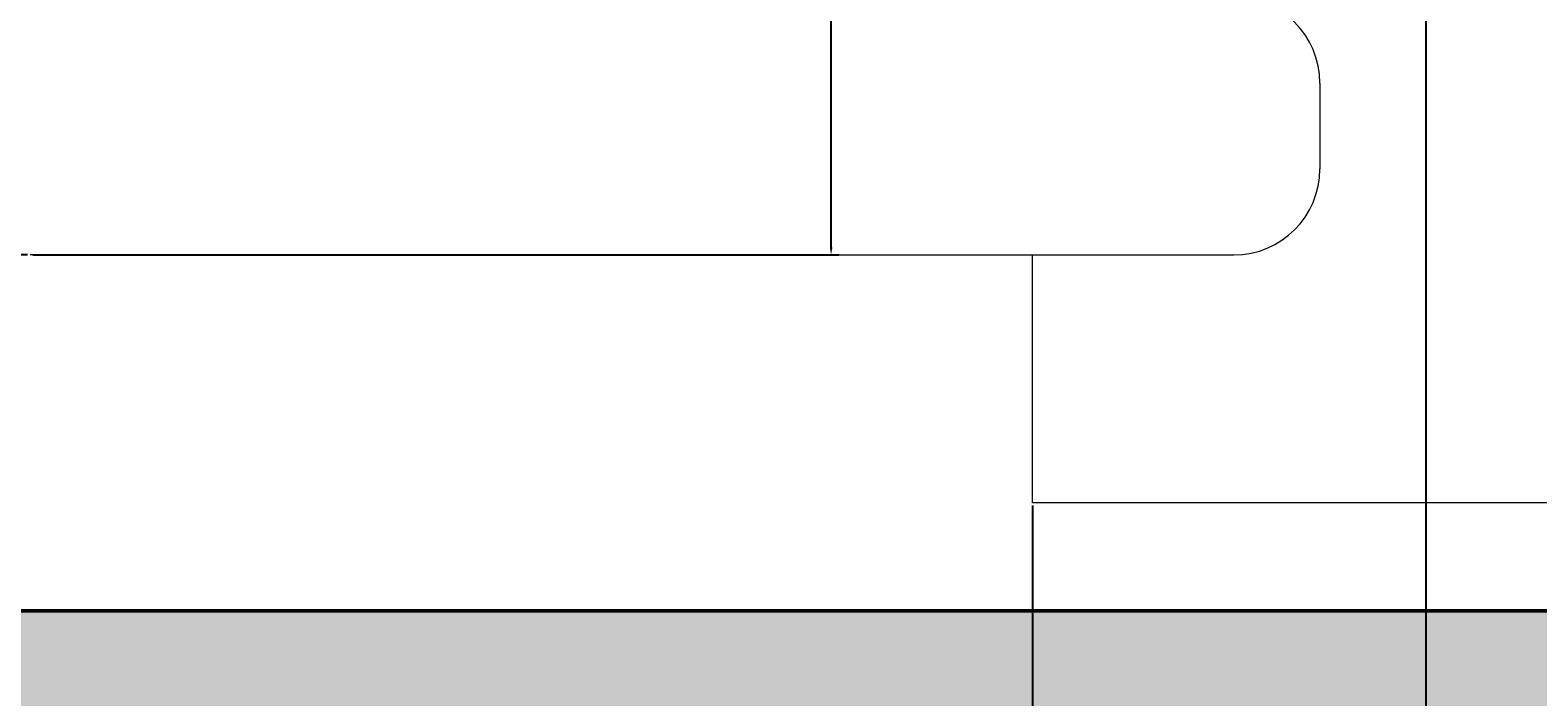
# Model space of a CAD drawing. Units: inches. Extents: x 2231 to 2461, y 2045 to 2455.
# Tile 38 of 95: x 2262 to 2297, y 2185 to 2200. Entities that reach past the tile are written whole.
import ezdxf

# ---------------------------------------------------------------- set-up
doc = ezdxf.new("R2010")
doc.units = ezdxf.units.IN
for name, color, linetype, lineweight in [('A-ANNO-DIMS', 2, 'Continuous', 18), ('A-FURN', 9, 'Continuous', 18), ('A-WALL', 7, 'Continuous', 50)]:
    doc.layers.add(name, color=color, linetype=linetype, lineweight=lineweight)
doc.layers.add('A-WALL-PATT', color=18, linetype='Continuous', lineweight=13, true_color=0x000000)
doc.styles.get("Standard").update_dxf_attribs({"font": 'arial.ttf'})
doc.dimstyles.get("Standard").update_dxf_attribs({"dimtxt": 0.18, "dimasz": 0.18, "dimexe": 0.18, "dimexo": 0.0625, "dimgap": 0.09, "dimtad": 0, "dimtih": 1, "dimtoh": 1, "dimdec": 4, "dimzin": 0, "dimdsep": 46, "dimtxsty": 'Standard', "dimcen": 0.09, "dimadec": 0, "dimazin": 0, "dimtfac": 1, "dimtdec": 4, "dimtofl": 0, "dimtmove": 0, "dimatfit": 3, "dimfxl": 1, "dimtolj": 1, "dimtzin": 0, "dimarcsym": 0})

# ---------------------------------------------------------------- blocks, each defined once
blk = doc.blocks.new('*D47')
at = {"layer": 'A-ANNO-DIMS', "color": 0, "lineweight": -2, "transparency": 16777216}
for p, q in [((2258.794, 2182.895), (2258.794, 2454.645)), ((2258.974, 2454.465), (2276.575, 2454.465)), ((2294.614, 2454.465), (2277.012, 2454.465)), ((2294.794, 2182.895), (2294.794, 2454.645))]:
    blk.add_line(p, q, dxfattribs=at)
at = {"layer": 'A-ANNO-DIMS', "color": 0, "transparency": 16777216}
for points in [[(2258.974, 2454.495), (2258.974, 2454.435), (2258.794, 2454.465)], [(2294.614, 2454.495), (2294.614, 2454.435), (2294.794, 2454.465)]]:
    blk.add_solid(points, dxfattribs=at)
at = {"layer": 'Defpoints', "color": 0, "transparency": 16777216}
for p in [(2294.794, 2454.465), (2258.794, 2182.833), (2294.794, 2182.833)]:
    blk.add_point(p, dxfattribs=at)
at = {"layer": 'A-ANNO-DIMS', "color": 0, "transparency": 16777216, "insert": (2276.794, 2454.465), "char_height": 0.18, "attachment_point": 5}
blk.add_mtext('\\A1;36', dxfattribs=at)
blk = doc.blocks.new('*D51')
at = {"layer": 'A-ANNO-DIMS', "color": 0, "lineweight": -2, "transparency": 16777216}
for p, q in [((2258.794, 2306.77), (2258.794, 2044.803)), ((2330.794, 2306.77), (2330.794, 2044.803)), ((2258.974, 2044.983), (2294.576, 2044.983)), ((2330.614, 2044.983), (2295.011, 2044.983))]:
    blk.add_line(p, q, dxfattribs=at)
at = {"layer": 'A-ANNO-DIMS', "color": 0, "transparency": 16777216}
for points in [[(2258.974, 2045.013), (2258.974, 2044.953), (2258.794, 2044.983)], [(2330.614, 2045.013), (2330.614, 2044.953), (2330.794, 2044.983)]]:
    blk.add_solid(points, dxfattribs=at)
at = {"layer": 'Defpoints', "color": 0, "transparency": 16777216}
for p in [(2258.794, 2306.833), (2330.794, 2306.833), (2330.794, 2044.983)]:
    blk.add_point(p, dxfattribs=at)
at = {"layer": 'A-ANNO-DIMS', "color": 0, "transparency": 16777216, "insert": (2294.794, 2044.983), "char_height": 0.18, "attachment_point": 5}
blk.add_mtext('\\A1;72', dxfattribs=at)
blk = doc.blocks.new('*D63')
at = {"layer": 'A-ANNO-DIMS', "color": 0, "lineweight": -2, "transparency": 16777216}
for p, q in [((2262.383, 2255.114), (2281.133, 2255.114)), ((2280.953, 2254.934), (2280.953, 2225.296)), ((2280.953, 2195.294), (2280.953, 2224.932)), ((2262.383, 2195.114), (2281.133, 2195.114))]:
    blk.add_line(p, q, dxfattribs=at)
at = {"layer": 'A-ANNO-DIMS', "color": 0, "transparency": 16777216}
for points in [[(2280.923, 2254.934), (2280.983, 2254.934), (2280.953, 2255.114)], [(2280.923, 2195.294), (2280.983, 2195.294), (2280.953, 2195.114)]]:
    blk.add_solid(points, dxfattribs=at)
at = {"layer": 'Defpoints', "color": 0, "transparency": 16777216}
for p in [(2262.321, 2255.114), (2262.321, 2195.114), (2280.953, 2195.114)]:
    blk.add_point(p, dxfattribs=at)
at = {"layer": 'A-ANNO-DIMS', "color": 0, "transparency": 16777216, "insert": (2280.953, 2225.114), "char_height": 0.18, "attachment_point": 5}
blk.add_mtext('\\A1;60', dxfattribs=at)
blk = doc.blocks.new('*D65')
at = {"layer": 'A-ANNO-DIMS', "color": 0, "lineweight": -2, "transparency": 16777216}
for p, q in [((2285.635, 2189.285), (2285.635, 2044.803)), ((2340.667, 2189.285), (2340.667, 2044.803)), ((2285.815, 2044.983), (2312.758, 2044.983)), ((2340.487, 2044.983), (2313.545, 2044.983))]:
    blk.add_line(p, q, dxfattribs=at)
at = {"layer": 'A-ANNO-DIMS', "color": 0, "transparency": 16777216}
for points in [[(2285.815, 2045.013), (2285.815, 2044.953), (2285.635, 2044.983)], [(2340.487, 2045.013), (2340.487, 2044.953), (2340.667, 2044.983)]]:
    blk.add_solid(points, dxfattribs=at)
at = {"layer": 'Defpoints', "color": 0, "transparency": 16777216}
for p in [(2285.635, 2189.348), (2340.667, 2189.348), (2340.667, 2044.983)]:
    blk.add_point(p, dxfattribs=at)
at = {"layer": 'A-ANNO-DIMS', "color": 0, "transparency": 16777216, "insert": (2313.151, 2044.983), "char_height": 0.18, "attachment_point": 5}
blk.add_mtext('\\A1;55.03', dxfattribs=at)
blk = doc.blocks.new('*D75')
at = {"layer": 'A-ANNO-DIMS', "color": 0, "lineweight": -2, "transparency": 16777216}
for p, q in [((2262.258, 2195.114), (2230.981, 2195.114)), ((2231.161, 2194.934), (2231.161, 2191.155)), ((2231.161, 2187.013), (2231.161, 2190.791)), ((2258.731, 2186.833), (2230.981, 2186.833))]:
    blk.add_line(p, q, dxfattribs=at)
at = {"layer": 'A-ANNO-DIMS', "color": 0, "transparency": 16777216}
for points in [[(2231.131, 2194.934), (2231.191, 2194.934), (2231.161, 2195.114)], [(2231.131, 2187.013), (2231.191, 2187.013), (2231.161, 2186.833)]]:
    blk.add_solid(points, dxfattribs=at)
at = {"layer": 'Defpoints', "color": 0, "transparency": 16777216}
for p in [(2231.161, 2195.114), (2262.321, 2195.114), (2258.794, 2186.833)]:
    blk.add_point(p, dxfattribs=at)
at = {"layer": 'A-ANNO-DIMS', "color": 0, "transparency": 16777216, "insert": (2231.161, 2190.973), "char_height": 0.18, "attachment_point": 5}
blk.add_mtext('\\A1;8.281', dxfattribs=at)

msp = doc.modelspace()

# ---------------------------------------------------------------- hatches: boundary and pattern name
at = {"layer": 'A-WALL-PATT'}
h = msp.add_hatch(color=256, dxfattribs=at)
h.dxf.hatch_style = 1
h.paths.add_polyline_path([(2441.7935, 2269.1535), (2432.7935, 2269.1535), (2432.7935, 2186.8328), (2396.7935, 2186.8328), (2396.7935, 2286.8328), (2394.7935, 2286.8328), (2394.7935, 2186.8328), (2334.7935, 2186.8328), (2334.7935, 2182.8328), (2432.7935, 2182.8328), (2432.7935, 2072.8328), (2416.6639, 2072.8328), (2416.6639, 2063.8328), (2441.7935, 2063.8328)])
h.paths.add_polyline_path([(2368.6639, 2072.8328), (2367.04, 2072.8328), (2330.7942, 2072.8328), (2330.7397, 2063.8328), (2368.6639, 2063.8328)])
h.paths.add_polyline_path([(2300.7392, 2068.3328), (2300.7392, 2072.8328), (2298.7935, 2072.8328), (2294.7935, 2072.8328), (2258.7935, 2072.8328), (2258.7935, 2120.8328), (2294.7935, 2120.8328), (2298.7935, 2120.8328), (2298.7935, 2128.8328), (2294.7935, 2128.8328), (2294.7935, 2124.8328), (2258.7935, 2124.8328), (2258.7935, 2182.8328), (2294.7935, 2182.8328), (2294.7935, 2174.8328), (2298.7935, 2174.8328), (2298.7935, 2182.8328), (2304.7935, 2182.8328), (2304.7935, 2186.8328), (2258.7935, 2186.8328), (2258.7935, 2221.999), (2249.7935, 2221.999), (2249.7935, 2063.8328), (2300.7392, 2063.8328)])
h.paths.add_polyline_path([(2391.9338, 2435.8328), (2333.82, 2435.8328), (2333.82, 2426.8328), (2368.7935, 2426.8328), (2368.7935, 2374.9508), (2368.7935, 2370.8328), (2372.3935, 2370.8328), (2372.7935, 2370.8328), (2372.7935, 2426.8328), (2391.9338, 2426.8328)])
h.paths.add_polyline_path([(2441.7935, 2435.8328), (2415.9338, 2435.8328), (2415.9338, 2426.8328), (2432.7935, 2426.8328), (2432.7935, 2334.8328), (2372.7935, 2334.8328), (2372.7935, 2346.8328), (2368.7935, 2346.8328), (2368.7935, 2306.8328), (2360.7935, 2306.8328), (2360.7935, 2302.8328), (2368.7935, 2302.8328), (2372.7935, 2302.8328), (2372.7935, 2330.8328), (2432.7935, 2330.8328), (2432.7935, 2317.1535), (2441.7935, 2317.1535)])
h.paths.add_polyline_path([(2285.82, 2435.8328), (2249.7935, 2435.8328), (2249.7935, 2269.999), (2258.7935, 2269.999), (2258.7935, 2302.8328), (2318.8168, 2302.8328), (2330.7935, 2302.8328), (2330.7935, 2306.8328), (2258.7935, 2306.8328), (2258.7935, 2426.8328), (2285.82, 2426.8328)])

# ---------------------------------------------------------------- linework, layer by layer
at = {"layer": 'A-FURN'}
for p, q in [((2292.3207, 2199.1137), (2292.3207, 2197.1137)), ((2268.3207, 2195.1137), (2262.3207, 2195.1137)), ((2268.3207, 2195.1137), (2290.3207, 2195.1137))]:
    msp.add_line(p, q, dxfattribs=at)
msp.add_lwpolyline([(2285.6353, 2255.1137), (2285.6353, 2261.3584), (2340.6673, 2261.3584), (2340.6673, 2189.3477), (2285.6353, 2189.3477), (2285.6353, 2195.1137)], dxfattribs=at)
for centre, start, end in [((2290.3207, 2199.1137), 0, 90), ((2290.3207, 2197.1137), 270, 0)]:
    msp.add_arc(centre, 2, start, end, dxfattribs=at)
at = {"layer": 'A-WALL'}
msp.add_line((2258.7935, 2186.8328), (2304.7935, 2186.8328), dxfattribs=at)

# ---------------------------------------------------------------- dimensions: what is measured, and where the dimension line sits
at = {"layer": 'A-ANNO-DIMS'}
for base, p1, p2, override, picture, middle in [((2294.7935, 2454.4653), (2258.7935, 2182.8328), (2294.7935, 2182.8328), {"dimdec": 0, "dimlfac": 1, "dimrnd": 0, "dimzin": 0, "dimdsep": 46, "dimlunit": 2}, '*D47', (2276.7935, 2454.4653)), ((2330.7935, 2044.9825), (2258.7935, 2306.8328), (2330.7935, 2306.8328), {"dimdec": 0, "dimlfac": 1, "dimrnd": 0, "dimzin": 0, "dimdsep": 46, "dimlunit": 2}, '*D51', (2294.7935, 2044.9825)), ((2340.6673, 2044.9825), (2285.6353, 2189.3477), (2340.6673, 2189.3477), {"dimdec": 2, "dimlfac": 1, "dimrnd": 0, "dimzin": 0, "dimdsep": 46, "dimlunit": 2}, '*D65', (2313.1513, 2044.9825))]:
    dim = msp.add_linear_dim(base=base, p1=p1, p2=p2, dimstyle='Standard', override=override, dxfattribs=at)
    dim.commit()
    dim.dimension.update_dxf_attribs({"geometry": picture, "text_midpoint": middle})
for base, p1, angle, override, picture, middle in [((2280.9532, 2195.1137), (2262.3207, 2255.1137), 270, {"dimdec": 0, "dimlfac": 1, "dimrnd": 0, "dimzin": 0, "dimdsep": 46, "dimlunit": 2}, '*D63', (2280.9532, 2225.1137)), ((2231.161, 2195.1137), (2258.7935, 2186.8328), 90, {"dimdec": 3, "dimlfac": 1, "dimrnd": 0, "dimzin": 0, "dimdsep": 46, "dimlunit": 2}, '*D75', (2231.161, 2190.9733))]:
    dim = msp.add_linear_dim(base=base, p1=p1, p2=(2262.3207, 2195.1137), angle=angle, dimstyle='Standard', override=override, dxfattribs=at)
    dim.commit()
    dim.dimension.update_dxf_attribs({"geometry": picture, "text_midpoint": middle})

doc.saveas('drawing.dxf')
